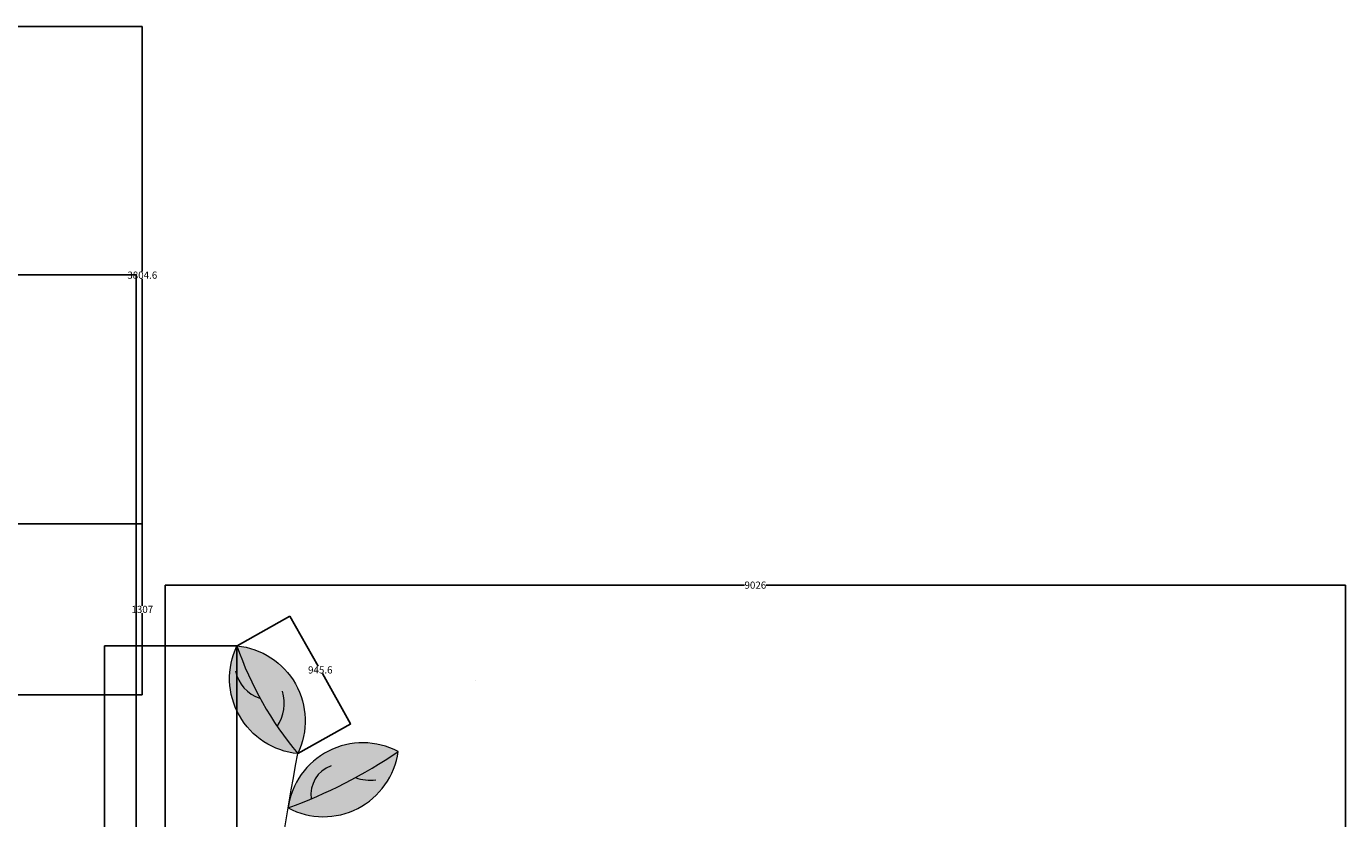
# Model space of a CAD drawing. Units: millimetres. Extents: x 8570 to 49085, y 3782 to 24863.
# Tile 15 of 15: x 35169 to 45255, y 15329 to 21387. Entities that reach past the tile are written whole.
import ezdxf

# ---------------------------------------------------------------- set-up
doc = ezdxf.new("R2010")
doc.units = ezdxf.units.MM
doc.header["$MEASUREMENT"] = 0
doc.header["$PDMODE"] = 3
for name, color, linetype, lineweight in [('A-ANNO-DIMS', 2, 'Continuous', 18), ('A-DETL-FOLI', 7, 'Continuous', 13), ('A-DETL-PATT', 3, 'Continuous', 13), ('A-DETL-STEM', 28, 'Continuous', 18)]:
    doc.layers.add(name, color=color, linetype=linetype, lineweight=lineweight)
doc.styles.get("Standard").update_dxf_attribs({"font": 'arial.ttf'})
doc.dimstyles.get("Standard").update_dxf_attribs({"dimtxt": 55, "dimasz": 0.18, "dimexe": 0.18, "dimexo": 0.0625, "dimgap": 0.09, "dimtad": 0, "dimtih": 1, "dimtoh": 1, "dimdec": 0, "dimzin": 0, "dimdsep": 46, "dimtxsty": 'Standard', "dimcen": 0.09, "dimadec": 0, "dimazin": 0, "dimtfac": 1, "dimtdec": 0, "dimtofl": 0, "dimtmove": 0, "dimatfit": 3, "dimfxl": 1, "dimtolj": 1, "dimtzin": 0, "dimarcsym": 0})

# ---------------------------------------------------------------- blocks, each defined once
blk = doc.blocks.new('*D15')
at = {"layer": 'A-ANNO-DIMS', "color": 0, "lineweight": -2, "transparency": 16777216}
for p, q in [((33971.06250000001, 19487.31685379339), (36009.05252806903, 19487.31685379339)), ((36008.87252806903, 19487.13685379339), (36008.87252806904, 12722.59869974799)), ((36008.87252806904, 5901.680000000003), (36008.87252806904, 12666.2181540454)), ((33971.06250000001, 5901.500000000002), (36009.05252806903, 5901.500000000003))]:
    blk.add_line(p, q, dxfattribs=at)
at = {"layer": 'A-ANNO-DIMS', "color": 0, "transparency": 16777216}
for points in [[(36008.84252806903, 19487.13685379339), (36008.90252806903, 19487.13685379339), (36008.87252806903, 19487.31685379339)], [(36008.84252806904, 5901.680000000003), (36008.90252806904, 5901.680000000003), (36008.87252806904, 5901.500000000003)]]:
    blk.add_solid(points, dxfattribs=at)
at = {"layer": 'Defpoints', "color": 0, "transparency": 16777216}
for p in [(33971.00000000002, 19487.31685379339), (36008.87252806903, 19487.31685379339), (33971.00000000002, 5901.500000000002)]:
    blk.add_point(p, dxfattribs=at)
at = {"layer": 'A-ANNO-DIMS', "color": 0, "transparency": 16777216, "insert": (36008.87252806903, 12694.40842689669), "char_height": 55, "attachment_point": 5}
blk.add_mtext('\\A1;MINARET 13586 TYP.', dxfattribs=at)
blk = doc.blocks.new('*D53')
at = {"layer": 'A-ANNO-DIMS', "color": 0, "lineweight": -2, "transparency": 16777216}
for p, q in [((26017.61772600001, 17582.816214), (36055.18000000003, 17582.816214)), ((36055.00000000003, 17582.636214), (36055.00000000003, 16957.5089928513)), ((36055.00000000004, 16276.00122600001), (36055.00000000003, 16901.12844714871)), ((25347.40117700001, 16275.82122600001), (36055.18000000004, 16275.82122600001))]:
    blk.add_line(p, q, dxfattribs=at)
at = {"layer": 'A-ANNO-DIMS', "color": 0, "transparency": 16777216}
for points in [[(36054.97000000003, 17582.636214), (36055.03000000003, 17582.636214), (36055.00000000003, 17582.816214)], [(36054.97000000004, 16276.00122600001), (36055.03000000004, 16276.00122600001), (36055.00000000004, 16275.82122600001)]]:
    blk.add_solid(points, dxfattribs=at)
at = {"layer": 'Defpoints', "color": 0, "transparency": 16777216}
for p in [(26017.55522600002, 17582.816214), (36055.00000000003, 17582.816214), (25347.33867700002, 16275.82122600001)]:
    blk.add_point(p, dxfattribs=at)
at = {"layer": 'A-ANNO-DIMS', "color": 0, "transparency": 16777216, "insert": (36055.00000000003, 16929.31871999999), "char_height": 55, "attachment_point": 5}
blk.add_mtext('\\A1;1307', dxfattribs=at)
blk = doc.blocks.new('*D54')
at = {"layer": 'A-ANNO-DIMS', "color": 0, "lineweight": -2, "transparency": 16777216}
for p, q in [((24765.69099400002, 21387.41061700001), (36055.18000000003, 21387.41061700001)), ((36055.00000000003, 21387.23061700001), (36055.00000000003, 19513.3036883513)), ((36055.00000000003, 17582.996214), (36055.00000000003, 19456.92314264871)), ((26017.61772600001, 17582.816214), (36055.18000000003, 17582.816214))]:
    blk.add_line(p, q, dxfattribs=at)
at = {"layer": 'A-ANNO-DIMS', "color": 0, "transparency": 16777216}
for points in [[(36054.97000000003, 21387.23061700001), (36055.03000000003, 21387.23061700001), (36055.00000000003, 21387.41061700001)], [(36054.97000000003, 17582.996214), (36055.03000000003, 17582.996214), (36055.00000000003, 17582.816214)]]:
    blk.add_solid(points, dxfattribs=at)
at = {"layer": 'Defpoints', "color": 0, "transparency": 16777216}
for p in [(24765.62849400002, 21387.41061700001), (36055.00000000003, 21387.41061700001), (26017.55522600002, 17582.816214)]:
    blk.add_point(p, dxfattribs=at)
at = {"layer": 'A-ANNO-DIMS', "color": 0, "transparency": 16777216, "insert": (36055.00000000003, 19485.11341549999), "char_height": 55, "attachment_point": 5}
blk.add_mtext('\\A1;3804.6', dxfattribs=at)
blk = doc.blocks.new('*D72')
at = {"layer": 'A-ANNO-DIMS', "color": 0, "lineweight": -2, "transparency": 16777216}
for p, q in [((36229.446171, 13941.825384), (36229.446171, 17114.807694)), ((36229.62617100001, 17114.627694), (40660.12544855865, 17114.627694)), ((45255.016868, 17114.627694), (40824.51759044134, 17114.627694)), ((45255.196868, 15109.551612), (45255.196868, 17114.807694))]:
    blk.add_line(p, q, dxfattribs=at)
at = {"layer": 'A-ANNO-DIMS', "color": 0, "transparency": 16777216}
for points in [[(36229.62617100001, 17114.657694), (36229.62617100001, 17114.597694), (36229.446171, 17114.627694)], [(45255.016868, 17114.657694), (45255.016868, 17114.597694), (45255.196868, 17114.627694)]]:
    blk.add_solid(points, dxfattribs=at)
at = {"layer": 'Defpoints', "color": 0, "transparency": 16777216}
for p in [(45255.196868, 17114.627694), (45255.196868, 15109.489112), (36229.446171, 13941.762884)]:
    blk.add_point(p, dxfattribs=at)
at = {"layer": 'A-ANNO-DIMS', "color": 0, "transparency": 16777216, "insert": (40742.3215195, 17114.627694), "char_height": 55, "attachment_point": 5}
blk.add_mtext('\\A1;9026', dxfattribs=at)
blk = doc.blocks.new('*D73')
at = {"layer": 'A-ANNO-DIMS', "color": 0, "lineweight": -2, "transparency": 16777216}
for p, q in [((36778.99867400002, 16650.127694), (35764.76617000003, 16650.127694)), ((35764.94617000002, 16649.947694), (35764.94617000003, 12094.98536132469)), ((35764.94617000003, 7483.680000000003), (35764.94617000003, 12038.64233267531)), ((39490.93750000002, 7483.500000000003), (35764.76617000003, 7483.500000000002))]:
    blk.add_line(p, q, dxfattribs=at)
at = {"layer": 'A-ANNO-DIMS', "color": 0, "transparency": 16777216}
for points in [[(35764.91617000003, 16649.947694), (35764.97617000002, 16649.947694), (35764.94617000002, 16650.127694)], [(35764.91617000003, 7483.680000000003), (35764.97617000003, 7483.680000000003), (35764.94617000003, 7483.500000000002)]]:
    blk.add_solid(points, dxfattribs=at)
at = {"layer": 'Defpoints', "color": 0, "transparency": 16777216}
for p in [(35764.94617000002, 16650.127694), (36779.06117400002, 16650.127694), (39491.00000000002, 7483.500000000003)]:
    blk.add_point(p, dxfattribs=at)
at = {"layer": 'A-ANNO-DIMS', "color": 0, "transparency": 16777216, "insert": (35764.94617000002, 12066.81384699999), "char_height": 55, "attachment_point": 5}
blk.add_mtext('\\A1;9167', dxfattribs=at)
blk = doc.blocks.new('*D74')
at = {"layer": 'A-ANNO-DIMS', "color": 0, "lineweight": -2, "transparency": 16777216}
for p, q in [((36779.061174, 16650.065194), (36779.061174, 7014.968942)), ((36229.446171, 13941.700384), (36229.446171, 7014.968942)), ((36229.62617100001, 7015.148942), (36411.38399992156, 7015.148942)), ((36778.881174, 7015.148942), (36597.12334507845, 7015.148942))]:
    blk.add_line(p, q, dxfattribs=at)
at = {"layer": 'A-ANNO-DIMS', "color": 0, "transparency": 16777216}
for points in [[(36229.62617100001, 7015.178942), (36229.62617100001, 7015.118942), (36229.446171, 7015.148942)], [(36778.881174, 7015.178942), (36778.881174, 7015.118942), (36779.061174, 7015.148942)]]:
    blk.add_solid(points, dxfattribs=at)
at = {"layer": 'Defpoints', "color": 0, "transparency": 16777216}
for p in [(36779.061174, 16650.127694), (36229.446171, 13941.762884), (36779.061174, 7015.148942)]:
    blk.add_point(p, dxfattribs=at)
at = {"layer": 'A-ANNO-DIMS', "color": 0, "transparency": 16777216, "insert": (36504.2536725, 7015.148942), "char_height": 55, "attachment_point": 5}
blk.add_mtext('\\A1;549.6', dxfattribs=at)
blk = doc.blocks.new('*D75')
at = {"layer": 'A-ANNO-DIMS', "color": 0, "lineweight": -2, "transparency": 16777216}
for p, q in [((36779.061174, 16650.065194), (36779.061174, 7014.968942)), ((39491, 7483.4375), (39491, 7014.968942)), ((36779.241174, 7015.148942), (38052.62817226603, 7015.148942)), ((39490.82, 7015.148942), (38217.43300173398, 7015.148942))]:
    blk.add_line(p, q, dxfattribs=at)
at = {"layer": 'A-ANNO-DIMS', "color": 0, "transparency": 16777216}
for points in [[(36779.241174, 7015.178942), (36779.241174, 7015.118942), (36779.061174, 7015.148942)], [(39490.82, 7015.178942), (39490.82, 7015.118942), (39491, 7015.148942)]]:
    blk.add_solid(points, dxfattribs=at)
at = {"layer": 'Defpoints', "color": 0, "transparency": 16777216}
for p in [(36779.061174, 16650.127694), (39491, 7483.500000000001), (39491, 7015.148942)]:
    blk.add_point(p, dxfattribs=at)
at = {"layer": 'A-ANNO-DIMS', "color": 0, "transparency": 16777216, "insert": (38135.030587, 7015.148942), "char_height": 55, "attachment_point": 5}
blk.add_mtext('\\A1;2712', dxfattribs=at)
blk = doc.blocks.new('*D77')
at = {"layer": 'A-ANNO-DIMS', "color": 0, "lineweight": -2, "transparency": 16777216}
for p, q in [((36779.11561169966, 16650.15839883438), (37183.79893811336, 16878.41445284423)), ((37183.73058746134, 16878.16924234615), (37400.03732378587, 16494.67128886919)), ((37648.12356905248, 16054.83030674284), (37431.81683272794, 16438.3282602198)), ((37243.68545269966, 15826.50590183438), (37648.36877955056, 16054.76195609082))]:
    blk.add_line(p, q, dxfattribs=at)
at = {"layer": 'A-ANNO-DIMS', "color": 0, "transparency": 16777216}
for points in [[(37183.75671755719, 16878.18398066665), (37183.7044573655, 16878.15450402564), (37183.64215753831, 16878.32602292119)], [(37648.14969914832, 16054.84504506334), (37648.09743895664, 16054.81556842233), (37648.21199897551, 16054.67352616779)]]:
    blk.add_solid(points, dxfattribs=at)
at = {"layer": 'Defpoints', "color": 0, "transparency": 16777216}
for p in [(36779.061174, 16650.127694), (37648.21199897551, 16054.67352616779), (37243.63101499999, 15826.47519699999)]:
    blk.add_point(p, dxfattribs=at)
at = {"layer": 'A-ANNO-DIMS', "color": 0, "transparency": 16777216, "insert": (37415.92707825692, 16466.49977454449), "char_height": 55, "attachment_point": 5}
blk.add_mtext('\\A1;945.6', dxfattribs=at)
blk = doc.blocks.new('*D97')
at = {"layer": 'A-ANNO-DIMS', "color": 0, "lineweight": -2, "transparency": 16777216}
for p, q in [((38605.21914800002, 16386.91816000001), (38605.39914800002, 16386.91816)), ((38605.30914800002, 16386.82816), (38605.30914800002, 16387.00816)), ((35838.58225699724, 9611.040480483021), (36876.03679714131, 12151.82796656842)), ((35838.40225699723, 9611.040480483021), (35838.58225699724, 9611.040480483021))]:
    blk.add_line(p, q, dxfattribs=at)
at = {"layer": 'A-ANNO-DIMS', "color": 0, "transparency": 16777216}
blk.add_solid([(36876.00902323605, 12151.83930721153), (36876.06457104658, 12151.8166259253), (36876.10484100002, 12151.99461000001)], dxfattribs=at)
at = {"layer": 'Defpoints', "color": 0, "transparency": 16777216}
for p in [(38605.30914800002, 16386.91816), (36876.10484100002, 12151.99461000001)]:
    blk.add_point(p, dxfattribs=at)
at = {"layer": 'A-ANNO-DIMS', "color": 0, "transparency": 16777216, "insert": (35670.42344390037, 9611.040480483021), "char_height": 55, "attachment_point": 5}
blk.add_mtext('\\A1;2X R4574', dxfattribs=at)

msp = doc.modelspace()

# ---------------------------------------------------------------- hatches: boundary and pattern name
at = {"layer": 'A-DETL-PATT'}
h = msp.add_hatch(color=256, dxfattribs=at)
h.dxf.hatch_style = 1
h.paths.add_polyline_path([(36779.06117360296, 16650.1276936674, 0.5205670500000067), (37243.63101477401, 15826.47519738877, -0.0921741816858173)])
h = msp.add_hatch(color=256, dxfattribs=at)
h.dxf.hatch_style = 1
h.paths.add_polyline_path([(36779.06117360296, 16650.12769366739, 0.0921741816858165), (37243.63101477401, 15826.47519738877, 0.5205670499999988)])
h = msp.add_hatch(color=256, dxfattribs=at)
h.dxf.hatch_style = 1
h.paths.add_polyline_path([(38011.23567257538, 15841.92330933591, 0.5205670500000026), (37169.4616527026, 15411.05781823815, 0.0631798539355979)])
h = msp.add_hatch(color=256, dxfattribs=at)
h.dxf.hatch_style = 1
h.paths.add_polyline_path([(38011.23567257538, 15841.9233093359, -0.0631798539355971), (37169.46165270261, 15411.05781823815, 0.5205670499999914)])

# ---------------------------------------------------------------- linework, layer by layer
at = {"layer": 'A-DETL-FOLI'}
for points in [[(37243.63101477401, 15826.47519738877, -0.52056705), (36779.06117360295, 16650.12769366739, -0.52056705)], [(37169.4616527026, 15411.05781823816, 0.52056705), (38011.23567257538, 15841.92330933591, 0.52056705)]]:
    msp.add_lwpolyline(points, format="xyb", close=True, dxfattribs=at)
for centre, radius, start, end in [((39226.32284806834, 17487.62856272467), 2586.599584199072, 198.8919509223256, 219.9571945175533), ((37032.20270418754, 16506.5053423219), 267.6964289322054, 190.3572477954385, 253.2192681205078), ((36821.8828197971, 16213.00901868681), 318.7731154335113, 326.0245460369875, 16.38170844288653), ((35892.23770956524, 18944.05883669977), 3756.7801635675, 289.8755553951192, 304.336091078083), ((37574.95246810131, 15514.93993171563), 230.4499337656383, 109.1571631303658, 188.6139861477091), ((37798.01610579441, 15973.50951094543), 349.8590159985452, 251.1090252995102, 277.0227011160281)]:
    msp.add_arc(centre, radius, start, end, dxfattribs=at)
at = {"layer": 'A-DETL-STEM'}
msp.add_open_spline([(39490.99999999999, 7483.500000000001), (38190.26814211403, 9726.554834160623), (36625.54732150807, 12424.84701443847), (37154.40566335566, 15335.42281512234), (37243.631014774, 15826.47519738878)], degree=3, knots=[0, 0, 0, 0, 7301.144293876133, 8782.942019613358, 8782.942019613358, 8782.942019613358, 8782.942019613358], dxfattribs=at)

# ---------------------------------------------------------------- dimensions: what is measured, and where the dimension line sits
at = {"layer": 'A-ANNO-DIMS'}
for base, p1, p2, angle, override, picture, middle in [((36055.00000000003, 21387.41061700001), (26017.555226, 17582.816214), (24765.628494, 21387.410617), 90, {"dimdec": 1, "dimlfac": 1, "dimrnd": 0, "dimzin": 0, "dimdsep": 46, "dimlunit": 2}, '*D54', (36055.00000000003, 19485.11341549999)), ((36055.00000000003, 17582.816214), (25347.338677, 16275.821226), (26017.555226, 17582.816214), 90, {"dimdec": 0, "dimlfac": 1, "dimrnd": 0, "dimzin": 0, "dimdsep": 46, "dimlunit": 2}, '*D53', (36055.00000000003, 16929.31871999999)), ((37648.21199897551, 16054.67352616779), (36779.061174, 16650.127694), (37243.631015, 15826.475197), 299.4245727199441, {"dimdec": 1, "dimlfac": 1, "dimrnd": 0, "dimzin": 0, "dimdsep": 46, "dimlunit": 2}, '*D77', (37415.92707825692, 16466.49977454449)), ((35764.94617000002, 16650.127694), (39491, 7483.500000000001), (36779.061174, 16650.127694), 90, {"dimdec": 0, "dimlfac": 1, "dimrnd": 0, "dimzin": 0, "dimdsep": 46, "dimlunit": 2}, '*D73', (35764.94617000002, 12066.81384699999))]:
    dim = msp.add_linear_dim(base=base, p1=p1, p2=p2, angle=angle, dimstyle='Standard', override=override, dxfattribs=at)
    dim.commit()
    dim.dimension.update_dxf_attribs({"geometry": picture, "text_midpoint": middle})
dim = msp.add_linear_dim(base=(36008.87252806903, 19487.31685379339), p1=(33971, 5901.5), p2=(33971, 19487.31685379339), angle=90, text='MINARET <> TYP.', dimstyle='Standard', override={"dimdec": 0, "dimlfac": 1, "dimrnd": 0, "dimzin": 0, "dimdsep": 46, "dimlunit": 2}, dxfattribs=at)
dim.commit()
dim.dimension.update_dxf_attribs({"geometry": '*D15', "text_midpoint": (36008.87252806903, 12694.40842689669)})
for base, p1, p2, override, picture, middle in [((45255.196868, 17114.627694), (36229.446171, 13941.762884), (45255.196868, 15109.489112), {"dimdec": 0, "dimlfac": 1, "dimrnd": 0, "dimzin": 0, "dimdsep": 46, "dimlunit": 2}, '*D72', (40742.3215195, 17114.627694)), ((36779.061174, 7015.148942), (36229.446171, 13941.762884), (36779.061174, 16650.127694), {"dimdec": 1, "dimlfac": 1, "dimrnd": 0, "dimzin": 0, "dimdsep": 46, "dimlunit": 2}, '*D74', (36504.2536725, 7015.148942)), ((39491, 7015.148942), (36779.061174, 16650.127694), (39491, 7483.500000000001), {"dimdec": 0, "dimlfac": 1, "dimrnd": 0, "dimzin": 0, "dimdsep": 46, "dimlunit": 2}, '*D75', (38135.030587, 7015.148942))]:
    dim = msp.add_linear_dim(base=base, p1=p1, p2=p2, dimstyle='Standard', override=override, dxfattribs=at)
    dim.commit()
    dim.dimension.update_dxf_attribs({"geometry": picture, "text_midpoint": middle})
dim = msp.add_radius_dim(center=(38605.30914800002, 16386.91816), mpoint=(36876.10484100002, 12151.99461000001), text='2X <>', dimstyle='Standard', override={"dimdec": 0, "dimlfac": 1, "dimrnd": 0, "dimzin": 0, "dimdsep": 46, "dimlunit": 2}, dxfattribs=at)
dim.commit()
dim.dimension.update_dxf_attribs({"geometry": '*D97', "text_midpoint": (35670.42344390037, 9611.040480483021), "dimtype": 164})

doc.saveas('drawing.dxf')
